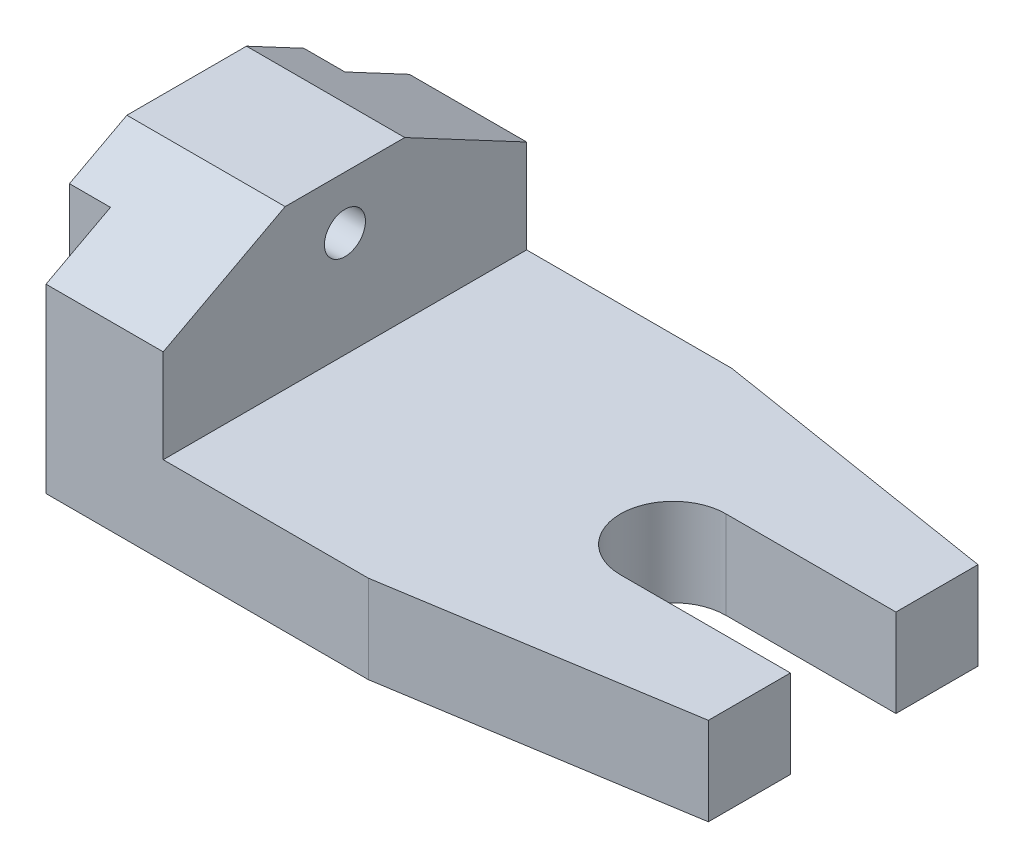
ISO-10303-21;
HEADER;
FILE_DESCRIPTION(('STEP AP214'),'2;1');
FILE_NAME('part.step','',(''),(''),'','','');
FILE_SCHEMA(('AUTOMOTIVE_DESIGN { 1 0 10303 214 1 1 1 1 }'));
ENDSEC;
DATA;
#1=APPLICATION_CONTEXT('core data for automotive mechanical design processes');
#2=APPLICATION_PROTOCOL_DEFINITION('international standard','automotive_design',2000,#1);
#3=PRODUCT_CONTEXT('',#1,'mechanical');
#4=PRODUCT('Part','Part','',(#3));
#5=PRODUCT_RELATED_PRODUCT_CATEGORY('part','',(#4));
#6=PRODUCT_DEFINITION_FORMATION('','',#4);
#7=PRODUCT_DEFINITION_CONTEXT('part definition',#1,'design');
#8=PRODUCT_DEFINITION('design','',#6,#7);
#9=PRODUCT_DEFINITION_SHAPE('','',#8);
#10=(LENGTH_UNIT() NAMED_UNIT(*) SI_UNIT(.MILLI.,.METRE.));
#11=(NAMED_UNIT(*) PLANE_ANGLE_UNIT() SI_UNIT($,.RADIAN.));
#12=(NAMED_UNIT(*) SI_UNIT($,.STERADIAN.) SOLID_ANGLE_UNIT());
#13=UNCERTAINTY_MEASURE_WITH_UNIT(LENGTH_MEASURE(1.E-05),#10,'distance_accuracy_value','');
#14=(GEOMETRIC_REPRESENTATION_CONTEXT(3) GLOBAL_UNCERTAINTY_ASSIGNED_CONTEXT((#13)) GLOBAL_UNIT_ASSIGNED_CONTEXT((#10,
#11,#12)) REPRESENTATION_CONTEXT('',''));
#15=CARTESIAN_POINT('',(0.,0.,0.));
#16=DIRECTION('',(0.,0.,1.));
#17=DIRECTION('',(1.,0.,0.));
#18=AXIS2_PLACEMENT_3D('',#15,#16,#17);
#19=CARTESIAN_POINT('',(112.,0.,31.));
#20=DIRECTION('',(-1.,0.,0.));
#21=DIRECTION('',(0.,0.,1.));
#22=AXIS2_PLACEMENT_3D('',#19,#20,#21);
#23=PLANE('',#22);
#24=DIRECTION('',(0.,0.,-1.));
#25=VECTOR('',#24,1.);
#26=CARTESIAN_POINT('',(112.,15.,31.));
#27=LINE('',#26,#25);
#28=CARTESIAN_POINT('',(112.,15.,23.));
#29=VERTEX_POINT('',#28);
#30=CARTESIAN_POINT('',(112.,15.,9.));
#31=VERTEX_POINT('',#30);
#32=EDGE_CURVE('E177',#29,#31,#27,.T.);
#33=ORIENTED_EDGE('',*,*,#32,.F.);
#34=DIRECTION('',(0.,1.,0.));
#35=VECTOR('',#34,1.);
#36=CARTESIAN_POINT('',(112.,-87.,23.));
#37=LINE('',#36,#35);
#38=CARTESIAN_POINT('',(112.,0.,23.));
#39=VERTEX_POINT('',#38);
#40=EDGE_CURVE('E165',#39,#29,#37,.T.);
#41=ORIENTED_EDGE('',*,*,#40,.F.);
#42=DIRECTION('',(0.,0.,-1.));
#43=VECTOR('',#42,1.);
#44=CARTESIAN_POINT('',(112.,0.,31.));
#45=LINE('',#44,#43);
#46=CARTESIAN_POINT('',(112.,0.,9.));
#47=VERTEX_POINT('',#46);
#48=EDGE_CURVE('E188',#39,#47,#45,.T.);
#49=ORIENTED_EDGE('',*,*,#48,.T.);
#50=DIRECTION('',(0.,1.,0.));
#51=VECTOR('',#50,1.);
#52=CARTESIAN_POINT('',(112.,-87.,9.));
#53=LINE('',#52,#51);
#54=EDGE_CURVE('E184',#47,#31,#53,.T.);
#55=ORIENTED_EDGE('',*,*,#54,.T.);
#56=EDGE_LOOP('',(#33,#41,#49,#55));
#57=FACE_BOUND('',#56,.T.);
#58=ADVANCED_FACE('F41',(#57),#23,.F.);
#59=CARTESIAN_POINT('',(0.,0.,31.));
#60=DIRECTION('',(0.,1.,0.));
#61=DIRECTION('',(0.,0.,1.));
#62=AXIS2_PLACEMENT_3D('',#59,#60,#61);
#63=PLANE('',#62);
#64=ORIENTED_EDGE('',*,*,#48,.F.);
#65=DIRECTION('',(-0.987440631916705,0.,0.157990501106673));
#66=VECTOR('',#65,1.);
#67=CARTESIAN_POINT('',(1.54758190327613,0.,40.6723868954758));
#68=LINE('',#67,#66);
#69=CARTESIAN_POINT('',(62.,0.,31.));
#70=VERTEX_POINT('',#69);
#71=EDGE_CURVE('E170',#39,#70,#68,.T.);
#72=ORIENTED_EDGE('',*,*,#71,.T.);
#73=DIRECTION('',(1.,0.,0.));
#74=VECTOR('',#73,1.);
#75=CARTESIAN_POINT('',(0.,0.,31.));
#76=LINE('',#75,#74);
#77=CARTESIAN_POINT('',(7.,0.,31.));
#78=VERTEX_POINT('',#77);
#79=EDGE_CURVE('E250',#78,#70,#76,.T.);
#80=ORIENTED_EDGE('',*,*,#79,.F.);
#81=DIRECTION('',(0.,0.,-1.));
#82=VECTOR('',#81,1.);
#83=CARTESIAN_POINT('',(7.,0.,31.));
#84=LINE('',#83,#82);
#85=CARTESIAN_POINT('',(7.,0.,20.));
#86=VERTEX_POINT('',#85);
#87=EDGE_CURVE('E297',#78,#86,#84,.T.);
#88=ORIENTED_EDGE('',*,*,#87,.T.);
#89=DIRECTION('',(-1.,0.,0.));
#90=VECTOR('',#89,1.);
#91=CARTESIAN_POINT('',(0.,0.,20.));
#92=LINE('',#91,#90);
#93=CARTESIAN_POINT('',(0.,0.,20.));
#94=VERTEX_POINT('',#93);
#95=EDGE_CURVE('E314',#86,#94,#92,.T.);
#96=ORIENTED_EDGE('',*,*,#95,.T.);
#97=DIRECTION('',(0.,0.,-1.));
#98=VECTOR('',#97,1.);
#99=CARTESIAN_POINT('',(0.,0.,31.));
#100=LINE('',#99,#98);
#101=CARTESIAN_POINT('',(0.,0.,-20.));
#102=VERTEX_POINT('',#101);
#103=EDGE_CURVE('E247',#94,#102,#100,.T.);
#104=ORIENTED_EDGE('',*,*,#103,.T.);
#105=DIRECTION('',(1.,0.,0.));
#106=VECTOR('',#105,1.);
#107=CARTESIAN_POINT('',(0.,0.,-20.));
#108=LINE('',#107,#106);
#109=CARTESIAN_POINT('',(7.,0.,-20.));
#110=VERTEX_POINT('',#109);
#111=EDGE_CURVE('E319',#102,#110,#108,.T.);
#112=ORIENTED_EDGE('',*,*,#111,.T.);
#113=DIRECTION('',(0.,0.,-1.));
#114=VECTOR('',#113,1.);
#115=CARTESIAN_POINT('',(7.00000000000002,0.,31.));
#116=LINE('',#115,#114);
#117=CARTESIAN_POINT('',(7.,0.,-31.));
#118=VERTEX_POINT('',#117);
#119=EDGE_CURVE('E232',#110,#118,#116,.T.);
#120=ORIENTED_EDGE('',*,*,#119,.T.);
#121=DIRECTION('',(1.,0.,0.));
#122=VECTOR('',#121,1.);
#123=CARTESIAN_POINT('',(0.,0.,-31.));
#124=LINE('',#123,#122);
#125=CARTESIAN_POINT('',(62.,0.,-31.));
#126=VERTEX_POINT('',#125);
#127=EDGE_CURVE('E224',#118,#126,#124,.T.);
#128=ORIENTED_EDGE('',*,*,#127,.T.);
#129=DIRECTION('',(0.987440631916706,0.,0.157990501106673));
#130=VECTOR('',#129,1.);
#131=CARTESIAN_POINT('',(11.2199687987519,0.,-39.1248049921997));
#132=LINE('',#131,#130);
#133=CARTESIAN_POINT('',(112.,0.,-23.));
#134=VERTEX_POINT('',#133);
#135=EDGE_CURVE('E175',#126,#134,#132,.T.);
#136=ORIENTED_EDGE('',*,*,#135,.T.);
#137=CARTESIAN_POINT('',(112.,0.,-9.));
#138=VERTEX_POINT('',#137);
#139=EDGE_CURVE('E187',#138,#134,#45,.T.);
#140=ORIENTED_EDGE('',*,*,#139,.F.);
#141=DIRECTION('',(-1.,0.,0.));
#142=VECTOR('',#141,1.);
#143=CARTESIAN_POINT('',(0.,0.,-8.99999999999999));
#144=LINE('',#143,#142);
#145=CARTESIAN_POINT('',(83.,0.,-9.));
#146=VERTEX_POINT('',#145);
#147=EDGE_CURVE('E288',#138,#146,#144,.T.);
#148=ORIENTED_EDGE('',*,*,#147,.T.);
#149=CARTESIAN_POINT('',(83.,0.,0.));
#150=DIRECTION('',(0.,1.,0.));
#151=DIRECTION('',(0.,0.,1.));
#152=AXIS2_PLACEMENT_3D('',#149,#150,#151);
#153=CIRCLE('',#152,9.);
#154=CARTESIAN_POINT('',(83.,0.,9.));
#155=VERTEX_POINT('',#154);
#156=EDGE_CURVE('E293',#146,#155,#153,.T.);
#157=ORIENTED_EDGE('',*,*,#156,.T.);
#158=DIRECTION('',(1.,0.,0.));
#159=VECTOR('',#158,1.);
#160=CARTESIAN_POINT('',(0.,0.,9.));
#161=LINE('',#160,#159);
#162=EDGE_CURVE('E295',#155,#47,#161,.T.);
#163=ORIENTED_EDGE('',*,*,#162,.T.);
#164=EDGE_LOOP('',(#64,#72,#80,#88,#96,#104,#112,#120,#128,#136,#140,#148,#157,#163));
#165=FACE_BOUND('',#164,.T.);
#166=ADVANCED_FACE('F43',(#165),#63,.F.);
#167=ORIENTED_EDGE('',*,*,#139,.T.);
#168=DIRECTION('',(0.,1.,0.));
#169=VECTOR('',#168,1.);
#170=CARTESIAN_POINT('',(112.,-87.,-23.));
#171=LINE('',#170,#169);
#172=CARTESIAN_POINT('',(112.,15.,-23.));
#173=VERTEX_POINT('',#172);
#174=EDGE_CURVE('E269',#134,#173,#171,.T.);
#175=ORIENTED_EDGE('',*,*,#174,.T.);
#176=CARTESIAN_POINT('',(112.,15.,-9.));
#177=VERTEX_POINT('',#176);
#178=EDGE_CURVE('E190',#177,#173,#27,.T.);
#179=ORIENTED_EDGE('',*,*,#178,.F.);
#180=DIRECTION('',(0.,1.,0.));
#181=VECTOR('',#180,1.);
#182=CARTESIAN_POINT('',(112.,-87.,-9.));
#183=LINE('',#182,#181);
#184=EDGE_CURVE('E57',#138,#177,#183,.T.);
#185=ORIENTED_EDGE('',*,*,#184,.F.);
#186=EDGE_LOOP('',(#167,#175,#179,#185));
#187=FACE_BOUND('',#186,.T.);
#188=ADVANCED_FACE('F350',(#187),#23,.F.);
#189=CARTESIAN_POINT('',(0.,15.,31.));
#190=DIRECTION('',(0.,1.,0.));
#191=DIRECTION('',(0.,0.,1.));
#192=AXIS2_PLACEMENT_3D('',#189,#190,#191);
#193=PLANE('',#192);
#194=DIRECTION('',(-0.987440631916705,0.,0.157990501106673));
#195=VECTOR('',#194,1.);
#196=CARTESIAN_POINT('',(62.,15.,31.));
#197=LINE('',#196,#195);
#198=CARTESIAN_POINT('',(62.,15.,31.));
#199=VERTEX_POINT('',#198);
#200=EDGE_CURVE('E64',#29,#199,#197,.T.);
#201=ORIENTED_EDGE('',*,*,#200,.F.);
#202=ORIENTED_EDGE('',*,*,#32,.T.);
#203=DIRECTION('',(1.,0.,0.));
#204=VECTOR('',#203,1.);
#205=CARTESIAN_POINT('',(83.,15.,9.));
#206=LINE('',#205,#204);
#207=CARTESIAN_POINT('',(83.,15.,9.));
#208=VERTEX_POINT('',#207);
#209=EDGE_CURVE('E273',#208,#31,#206,.T.);
#210=ORIENTED_EDGE('',*,*,#209,.F.);
#211=CARTESIAN_POINT('',(83.,15.,0.));
#212=DIRECTION('',(0.,1.,0.));
#213=DIRECTION('',(0.,0.,1.));
#214=AXIS2_PLACEMENT_3D('',#211,#212,#213);
#215=CIRCLE('',#214,9.);
#216=CARTESIAN_POINT('',(83.,15.,-9.));
#217=VERTEX_POINT('',#216);
#218=EDGE_CURVE('E285',#217,#208,#215,.T.);
#219=ORIENTED_EDGE('',*,*,#218,.F.);
#220=DIRECTION('',(-1.,0.,0.));
#221=VECTOR('',#220,1.);
#222=CARTESIAN_POINT('',(83.,15.,-9.));
#223=LINE('',#222,#221);
#224=EDGE_CURVE('E272',#177,#217,#223,.T.);
#225=ORIENTED_EDGE('',*,*,#224,.F.);
#226=ORIENTED_EDGE('',*,*,#178,.T.);
#227=DIRECTION('',(0.987440631916705,0.,0.157990501106673));
#228=VECTOR('',#227,1.);
#229=CARTESIAN_POINT('',(62.,15.,-31.));
#230=LINE('',#229,#228);
#231=CARTESIAN_POINT('',(62.,15.,-31.));
#232=VERTEX_POINT('',#231);
#233=EDGE_CURVE('E185',#232,#173,#230,.T.);
#234=ORIENTED_EDGE('',*,*,#233,.F.);
#235=DIRECTION('',(1.,0.,0.));
#236=VECTOR('',#235,1.);
#237=CARTESIAN_POINT('',(0.,15.,-31.));
#238=LINE('',#237,#236);
#239=CARTESIAN_POINT('',(27.,15.,-31.));
#240=VERTEX_POINT('',#239);
#241=EDGE_CURVE('E227',#240,#232,#238,.T.);
#242=ORIENTED_EDGE('',*,*,#241,.F.);
#243=DIRECTION('',(0.,0.,-1.));
#244=VECTOR('',#243,1.);
#245=CARTESIAN_POINT('',(27.,15.,31.));
#246=LINE('',#245,#244);
#247=CARTESIAN_POINT('',(27.,15.,31.));
#248=VERTEX_POINT('',#247);
#249=EDGE_CURVE('E194',#248,#240,#246,.T.);
#250=ORIENTED_EDGE('',*,*,#249,.F.);
#251=DIRECTION('',(1.,0.,0.));
#252=VECTOR('',#251,1.);
#253=CARTESIAN_POINT('',(0.,15.,31.));
#254=LINE('',#253,#252);
#255=EDGE_CURVE('E181',#248,#199,#254,.T.);
#256=ORIENTED_EDGE('',*,*,#255,.T.);
#257=EDGE_LOOP('',(#201,#202,#210,#219,#225,#226,#234,#242,#250,#256));
#258=FACE_BOUND('',#257,.T.);
#259=ADVANCED_FACE('F180',(#258),#193,.T.);
#260=CARTESIAN_POINT('',(27.,0.,31.));
#261=DIRECTION('',(-1.,0.,0.));
#262=DIRECTION('',(0.,0.,1.));
#263=AXIS2_PLACEMENT_3D('',#260,#261,#262);
#264=PLANE('',#263);
#265=CARTESIAN_POINT('',(27.,33.,0.));
#266=DIRECTION('',(-1.,0.,0.));
#267=DIRECTION('',(0.,0.,1.));
#268=AXIS2_PLACEMENT_3D('',#265,#266,#267);
#269=CIRCLE('',#268,3.5);
#270=CARTESIAN_POINT('',(27.,33.,3.5));
#271=VERTEX_POINT('',#270);
#272=EDGE_CURVE('E201',#271,#271,#269,.T.);
#273=ORIENTED_EDGE('',*,*,#272,.T.);
#274=EDGE_LOOP('',(#273));
#275=FACE_BOUND('',#274,.T.);
#276=DIRECTION('',(0.,0.,-1.));
#277=VECTOR('',#276,1.);
#278=CARTESIAN_POINT('',(27.,42.,31.));
#279=LINE('',#278,#277);
#280=CARTESIAN_POINT('',(27.,42.,10.2));
#281=VERTEX_POINT('',#280);
#282=CARTESIAN_POINT('',(27.,42.,-10.2029798390233));
#283=VERTEX_POINT('',#282);
#284=EDGE_CURVE('E254',#281,#283,#279,.T.);
#285=ORIENTED_EDGE('',*,*,#284,.F.);
#286=DIRECTION('',(0.,-0.469471562785885,0.88294759285893));
#287=VECTOR('',#286,1.);
#288=CARTESIAN_POINT('',(27.,24.1210602183135,43.8253952197516));
#289=LINE('',#288,#287);
#290=CARTESIAN_POINT('',(27.,30.9404438214414,31.));
#291=VERTEX_POINT('',#290);
#292=EDGE_CURVE('E207',#281,#291,#289,.T.);
#293=ORIENTED_EDGE('',*,*,#292,.T.);
#294=DIRECTION('',(0.,1.,0.));
#295=VECTOR('',#294,1.);
#296=CARTESIAN_POINT('',(27.,0.,31.));
#297=LINE('',#296,#295);
#298=EDGE_CURVE('E245',#248,#291,#297,.T.);
#299=ORIENTED_EDGE('',*,*,#298,.F.);
#300=ORIENTED_EDGE('',*,*,#249,.T.);
#301=DIRECTION('',(0.,1.,0.));
#302=VECTOR('',#301,1.);
#303=CARTESIAN_POINT('',(27.,0.,-31.));
#304=LINE('',#303,#302);
#305=CARTESIAN_POINT('',(27.,30.9420282299548,-31.));
#306=VERTEX_POINT('',#305);
#307=EDGE_CURVE('E240',#240,#306,#304,.T.);
#308=ORIENTED_EDGE('',*,*,#307,.T.);
#309=DIRECTION('',(0.,0.469471562785892,0.882947592858926));
#310=VECTOR('',#309,1.);
#311=CARTESIAN_POINT('',(27.,49.8224601667748,4.50892802074745));
#312=LINE('',#311,#310);
#313=EDGE_CURVE('E330',#306,#283,#312,.T.);
#314=ORIENTED_EDGE('',*,*,#313,.T.);
#315=EDGE_LOOP('',(#285,#293,#299,#300,#308,#314));
#316=FACE_BOUND('',#315,.T.);
#317=ADVANCED_FACE('F262',(#275,#316),#264,.F.);
#318=CARTESIAN_POINT('',(0.,42.,31.));
#319=DIRECTION('',(0.,1.,0.));
#320=DIRECTION('',(0.,0.,1.));
#321=AXIS2_PLACEMENT_3D('',#318,#319,#320);
#322=PLANE('',#321);
#323=DIRECTION('',(1.,0.,0.));
#324=VECTOR('',#323,1.);
#325=CARTESIAN_POINT('',(-4.,42.,10.2));
#326=LINE('',#325,#324);
#327=CARTESIAN_POINT('',(0.,42.,10.2));
#328=VERTEX_POINT('',#327);
#329=EDGE_CURVE('E322',#328,#281,#326,.T.);
#330=ORIENTED_EDGE('',*,*,#329,.T.);
#331=ORIENTED_EDGE('',*,*,#284,.T.);
#332=DIRECTION('',(1.,0.,0.));
#333=VECTOR('',#332,1.);
#334=CARTESIAN_POINT('',(-4.,42.,-10.2029798390233));
#335=LINE('',#334,#333);
#336=CARTESIAN_POINT('',(0.,42.,-10.2029798390233));
#337=VERTEX_POINT('',#336);
#338=EDGE_CURVE('E325',#337,#283,#335,.T.);
#339=ORIENTED_EDGE('',*,*,#338,.F.);
#340=DIRECTION('',(0.,0.,-1.));
#341=VECTOR('',#340,1.);
#342=CARTESIAN_POINT('',(0.,42.,31.));
#343=LINE('',#342,#341);
#344=EDGE_CURVE('E252',#328,#337,#343,.T.);
#345=ORIENTED_EDGE('',*,*,#344,.F.);
#346=EDGE_LOOP('',(#330,#331,#339,#345));
#347=FACE_BOUND('',#346,.T.);
#348=ADVANCED_FACE('F374',(#347),#322,.T.);
#349=CARTESIAN_POINT('',(0.,0.,31.));
#350=DIRECTION('',(-1.,0.,0.));
#351=DIRECTION('',(0.,0.,1.));
#352=AXIS2_PLACEMENT_3D('',#349,#350,#351);
#353=PLANE('',#352);
#354=DIRECTION('',(0.,1.,0.));
#355=VECTOR('',#354,1.);
#356=CARTESIAN_POINT('',(0.,-8.99999999999998,-20.));
#357=LINE('',#356,#355);
#358=CARTESIAN_POINT('',(0.,36.790831978231,-20.));
#359=VERTEX_POINT('',#358);
#360=EDGE_CURVE('E302',#102,#359,#357,.T.);
#361=ORIENTED_EDGE('',*,*,#360,.F.);
#362=ORIENTED_EDGE('',*,*,#103,.F.);
#363=DIRECTION('',(0.,1.,0.));
#364=VECTOR('',#363,1.);
#365=CARTESIAN_POINT('',(0.,-8.99999999999998,20.));
#366=LINE('',#365,#364);
#367=CARTESIAN_POINT('',(0.,36.7892475697176,20.));
#368=VERTEX_POINT('',#367);
#369=EDGE_CURVE('E300',#94,#368,#366,.T.);
#370=ORIENTED_EDGE('',*,*,#369,.T.);
#371=DIRECTION('',(0.,-0.469471562785885,0.88294759285893));
#372=VECTOR('',#371,1.);
#373=CARTESIAN_POINT('',(0.,24.1210602183135,43.8253952197516));
#374=LINE('',#373,#372);
#375=EDGE_CURVE('E326',#328,#368,#374,.T.);
#376=ORIENTED_EDGE('',*,*,#375,.F.);
#377=ORIENTED_EDGE('',*,*,#344,.T.);
#378=DIRECTION('',(0.,0.469471562785892,0.882947592858926));
#379=VECTOR('',#378,1.);
#380=CARTESIAN_POINT('',(0.,49.8224601667748,4.50892802074745));
#381=LINE('',#380,#379);
#382=EDGE_CURVE('E321',#359,#337,#381,.T.);
#383=ORIENTED_EDGE('',*,*,#382,.F.);
#384=EDGE_LOOP('',(#361,#362,#370,#376,#377,#383));
#385=FACE_BOUND('',#384,.T.);
#386=CARTESIAN_POINT('',(0.,33.,0.));
#387=DIRECTION('',(-1.,0.,0.));
#388=DIRECTION('',(0.,0.,1.));
#389=AXIS2_PLACEMENT_3D('',#386,#387,#388);
#390=CIRCLE('',#389,3.5);
#391=CARTESIAN_POINT('',(0.,33.,3.5));
#392=VERTEX_POINT('',#391);
#393=EDGE_CURVE('E205',#392,#392,#390,.T.);
#394=ORIENTED_EDGE('',*,*,#393,.F.);
#395=EDGE_LOOP('',(#394));
#396=FACE_BOUND('',#395,.T.);
#397=ADVANCED_FACE('F382',(#385,#396),#353,.T.);
#398=CARTESIAN_POINT('',(0.,0.,31.));
#399=DIRECTION('',(0.,0.,1.));
#400=DIRECTION('',(1.,0.,0.));
#401=AXIS2_PLACEMENT_3D('',#398,#399,#400);
#402=PLANE('',#401);
#403=DIRECTION('',(0.,-1.,0.));
#404=VECTOR('',#403,1.);
#405=CARTESIAN_POINT('',(62.,0.,31.));
#406=LINE('',#405,#404);
#407=EDGE_CURVE('E11',#199,#70,#406,.T.);
#408=ORIENTED_EDGE('',*,*,#407,.F.);
#409=ORIENTED_EDGE('',*,*,#255,.F.);
#410=ORIENTED_EDGE('',*,*,#298,.T.);
#411=DIRECTION('',(1.,0.,0.));
#412=VECTOR('',#411,1.);
#413=CARTESIAN_POINT('',(0.,30.9404438214414,31.));
#414=LINE('',#413,#412);
#415=CARTESIAN_POINT('',(7.,30.9404438214414,31.));
#416=VERTEX_POINT('',#415);
#417=EDGE_CURVE('E196',#416,#291,#414,.T.);
#418=ORIENTED_EDGE('',*,*,#417,.F.);
#419=DIRECTION('',(0.,1.,0.));
#420=VECTOR('',#419,1.);
#421=CARTESIAN_POINT('',(7.,-8.99999999999998,31.));
#422=LINE('',#421,#420);
#423=EDGE_CURVE('E306',#78,#416,#422,.T.);
#424=ORIENTED_EDGE('',*,*,#423,.F.);
#425=ORIENTED_EDGE('',*,*,#79,.T.);
#426=EDGE_LOOP('',(#408,#409,#410,#418,#424,#425));
#427=FACE_BOUND('',#426,.T.);
#428=ADVANCED_FACE('F337',(#427),#402,.T.);
#429=CARTESIAN_POINT('',(0.,0.,-31.));
#430=DIRECTION('',(0.,0.,1.));
#431=DIRECTION('',(1.,0.,0.));
#432=AXIS2_PLACEMENT_3D('',#429,#430,#431);
#433=PLANE('',#432);
#434=ORIENTED_EDGE('',*,*,#241,.T.);
#435=DIRECTION('',(0.,-1.,0.));
#436=VECTOR('',#435,1.);
#437=CARTESIAN_POINT('',(62.,0.,-31.));
#438=LINE('',#437,#436);
#439=EDGE_CURVE('E47',#232,#126,#438,.T.);
#440=ORIENTED_EDGE('',*,*,#439,.T.);
#441=ORIENTED_EDGE('',*,*,#127,.F.);
#442=DIRECTION('',(0.,1.,0.));
#443=VECTOR('',#442,1.);
#444=CARTESIAN_POINT('',(7.,-8.99999999999998,-31.));
#445=LINE('',#444,#443);
#446=CARTESIAN_POINT('',(7.,30.9420282299548,-31.));
#447=VERTEX_POINT('',#446);
#448=EDGE_CURVE('E296',#118,#447,#445,.T.);
#449=ORIENTED_EDGE('',*,*,#448,.T.);
#450=DIRECTION('',(1.,0.,0.));
#451=VECTOR('',#450,1.);
#452=CARTESIAN_POINT('',(0.,30.9420282299548,-31.));
#453=LINE('',#452,#451);
#454=EDGE_CURVE('E200',#447,#306,#453,.T.);
#455=ORIENTED_EDGE('',*,*,#454,.T.);
#456=ORIENTED_EDGE('',*,*,#307,.F.);
#457=EDGE_LOOP('',(#434,#440,#441,#449,#455,#456));
#458=FACE_BOUND('',#457,.T.);
#459=ADVANCED_FACE('F225',(#458),#433,.F.);
#460=CARTESIAN_POINT('',(-4.,42.,-10.2029798390233));
#461=DIRECTION('',(0.,-0.882947592858926,0.469471562785892));
#462=DIRECTION('',(0.,-0.469471562785892,-0.882947592858926));
#463=AXIS2_PLACEMENT_3D('',#460,#461,#462);
#464=PLANE('',#463);
#465=ORIENTED_EDGE('',*,*,#454,.F.);
#466=DIRECTION('',(0.,0.469471562785892,0.882947592858926));
#467=VECTOR('',#466,1.);
#468=CARTESIAN_POINT('',(7.,42.,-10.2029798390233));
#469=LINE('',#468,#467);
#470=CARTESIAN_POINT('',(7.,36.790831978231,-20.));
#471=VERTEX_POINT('',#470);
#472=EDGE_CURVE('E213',#447,#471,#469,.T.);
#473=ORIENTED_EDGE('',*,*,#472,.T.);
#474=DIRECTION('',(-1.,0.,0.));
#475=VECTOR('',#474,1.);
#476=CARTESIAN_POINT('',(-4.,36.790831978231,-20.));
#477=LINE('',#476,#475);
#478=EDGE_CURVE('E215',#471,#359,#477,.T.);
#479=ORIENTED_EDGE('',*,*,#478,.T.);
#480=ORIENTED_EDGE('',*,*,#382,.T.);
#481=ORIENTED_EDGE('',*,*,#338,.T.);
#482=ORIENTED_EDGE('',*,*,#313,.F.);
#483=EDGE_LOOP('',(#465,#473,#479,#480,#481,#482));
#484=FACE_BOUND('',#483,.T.);
#485=ADVANCED_FACE('F387',(#484),#464,.F.);
#486=CARTESIAN_POINT('',(-4.,42.,10.2));
#487=DIRECTION('',(0.,-0.88294759285893,-0.469471562785885));
#488=DIRECTION('',(0.,0.469471562785885,-0.88294759285893));
#489=AXIS2_PLACEMENT_3D('',#486,#487,#488);
#490=PLANE('',#489);
#491=ORIENTED_EDGE('',*,*,#375,.T.);
#492=DIRECTION('',(1.,0.,0.));
#493=VECTOR('',#492,1.);
#494=CARTESIAN_POINT('',(-4.,36.7892475697176,20.));
#495=LINE('',#494,#493);
#496=CARTESIAN_POINT('',(7.,36.7892475697176,20.));
#497=VERTEX_POINT('',#496);
#498=EDGE_CURVE('E209',#368,#497,#495,.T.);
#499=ORIENTED_EDGE('',*,*,#498,.T.);
#500=DIRECTION('',(0.,-0.469471562785885,0.88294759285893));
#501=VECTOR('',#500,1.);
#502=CARTESIAN_POINT('',(7.,42.,10.2));
#503=LINE('',#502,#501);
#504=EDGE_CURVE('E202',#497,#416,#503,.T.);
#505=ORIENTED_EDGE('',*,*,#504,.T.);
#506=ORIENTED_EDGE('',*,*,#417,.T.);
#507=ORIENTED_EDGE('',*,*,#292,.F.);
#508=ORIENTED_EDGE('',*,*,#329,.F.);
#509=EDGE_LOOP('',(#491,#499,#505,#506,#507,#508));
#510=FACE_BOUND('',#509,.T.);
#511=ADVANCED_FACE('F395',(#510),#490,.F.);
#512=CARTESIAN_POINT('',(-4.,33.,0.));
#513=DIRECTION('',(1.,0.,0.));
#514=DIRECTION('',(0.,0.,-1.));
#515=AXIS2_PLACEMENT_3D('',#512,#513,#514);
#516=CYLINDRICAL_SURFACE('',#515,3.5);
#517=ORIENTED_EDGE('',*,*,#393,.T.);
#518=EDGE_LOOP('',(#517));
#519=FACE_BOUND('',#518,.T.);
#520=ORIENTED_EDGE('',*,*,#272,.F.);
#521=EDGE_LOOP('',(#520));
#522=FACE_BOUND('',#521,.T.);
#523=ADVANCED_FACE('F389',(#519,#522),#516,.F.);
#524=CARTESIAN_POINT('',(0.,-8.99999999999998,20.));
#525=DIRECTION('',(0.,0.,-1.));
#526=DIRECTION('',(-1.,0.,0.));
#527=AXIS2_PLACEMENT_3D('',#524,#525,#526);
#528=PLANE('',#527);
#529=DIRECTION('',(0.,1.,0.));
#530=VECTOR('',#529,1.);
#531=CARTESIAN_POINT('',(7.,-8.99999999999998,20.));
#532=LINE('',#531,#530);
#533=EDGE_CURVE('E308',#86,#497,#532,.T.);
#534=ORIENTED_EDGE('',*,*,#533,.T.);
#535=ORIENTED_EDGE('',*,*,#498,.F.);
#536=ORIENTED_EDGE('',*,*,#369,.F.);
#537=ORIENTED_EDGE('',*,*,#95,.F.);
#538=EDGE_LOOP('',(#534,#535,#536,#537));
#539=FACE_BOUND('',#538,.T.);
#540=ADVANCED_FACE('F392',(#539),#528,.F.);
#541=CARTESIAN_POINT('',(7.,-8.99999999999998,31.));
#542=DIRECTION('',(1.,0.,0.));
#543=DIRECTION('',(0.,0.,-1.));
#544=AXIS2_PLACEMENT_3D('',#541,#542,#543);
#545=PLANE('',#544);
#546=ORIENTED_EDGE('',*,*,#423,.T.);
#547=ORIENTED_EDGE('',*,*,#504,.F.);
#548=ORIENTED_EDGE('',*,*,#533,.F.);
#549=ORIENTED_EDGE('',*,*,#87,.F.);
#550=EDGE_LOOP('',(#546,#547,#548,#549));
#551=FACE_BOUND('',#550,.T.);
#552=ADVANCED_FACE('F405',(#551),#545,.F.);
#553=CARTESIAN_POINT('',(7.,-8.99999999999998,-31.));
#554=DIRECTION('',(1.,0.,0.));
#555=DIRECTION('',(0.,0.,-1.));
#556=AXIS2_PLACEMENT_3D('',#553,#554,#555);
#557=PLANE('',#556);
#558=DIRECTION('',(0.,1.,0.));
#559=VECTOR('',#558,1.);
#560=CARTESIAN_POINT('',(7.,-8.99999999999998,-20.));
#561=LINE('',#560,#559);
#562=EDGE_CURVE('E301',#110,#471,#561,.T.);
#563=ORIENTED_EDGE('',*,*,#562,.T.);
#564=ORIENTED_EDGE('',*,*,#472,.F.);
#565=ORIENTED_EDGE('',*,*,#448,.F.);
#566=ORIENTED_EDGE('',*,*,#119,.F.);
#567=EDGE_LOOP('',(#563,#564,#565,#566));
#568=FACE_BOUND('',#567,.T.);
#569=ADVANCED_FACE('F356',(#568),#557,.F.);
#570=CARTESIAN_POINT('',(0.,-8.99999999999998,-20.));
#571=DIRECTION('',(0.,0.,1.));
#572=DIRECTION('',(1.,0.,0.));
#573=AXIS2_PLACEMENT_3D('',#570,#571,#572);
#574=PLANE('',#573);
#575=ORIENTED_EDGE('',*,*,#360,.T.);
#576=ORIENTED_EDGE('',*,*,#478,.F.);
#577=ORIENTED_EDGE('',*,*,#562,.F.);
#578=ORIENTED_EDGE('',*,*,#111,.F.);
#579=EDGE_LOOP('',(#575,#576,#577,#578));
#580=FACE_BOUND('',#579,.T.);
#581=ADVANCED_FACE('F348',(#580),#574,.F.);
#582=CARTESIAN_POINT('',(62.,-87.,-31.));
#583=DIRECTION('',(-0.157990501106673,0.,0.987440631916705));
#584=DIRECTION('',(0.987440631916706,0.,0.157990501106673));
#585=AXIS2_PLACEMENT_3D('',#582,#583,#584);
#586=PLANE('',#585);
#587=ORIENTED_EDGE('',*,*,#439,.F.);
#588=ORIENTED_EDGE('',*,*,#233,.T.);
#589=ORIENTED_EDGE('',*,*,#174,.F.);
#590=ORIENTED_EDGE('',*,*,#135,.F.);
#591=EDGE_LOOP('',(#587,#588,#589,#590));
#592=FACE_BOUND('',#591,.T.);
#593=ADVANCED_FACE('F349',(#592),#586,.F.);
#594=CARTESIAN_POINT('',(62.,-87.,31.));
#595=DIRECTION('',(-0.157990501106673,0.,-0.987440631916706));
#596=DIRECTION('',(-0.987440631916705,0.,0.157990501106673));
#597=AXIS2_PLACEMENT_3D('',#594,#595,#596);
#598=PLANE('',#597);
#599=ORIENTED_EDGE('',*,*,#40,.T.);
#600=ORIENTED_EDGE('',*,*,#200,.T.);
#601=ORIENTED_EDGE('',*,*,#407,.T.);
#602=ORIENTED_EDGE('',*,*,#71,.F.);
#603=EDGE_LOOP('',(#599,#600,#601,#602));
#604=FACE_BOUND('',#603,.T.);
#605=ADVANCED_FACE('F164',(#604),#598,.F.);
#606=CARTESIAN_POINT('',(83.,-87.,9.));
#607=DIRECTION('',(0.,0.,1.));
#608=DIRECTION('',(1.,0.,0.));
#609=AXIS2_PLACEMENT_3D('',#606,#607,#608);
#610=PLANE('',#609);
#611=DIRECTION('',(0.,1.,0.));
#612=VECTOR('',#611,1.);
#613=CARTESIAN_POINT('',(83.,-87.,9.));
#614=LINE('',#613,#612);
#615=EDGE_CURVE('E279',#155,#208,#614,.T.);
#616=ORIENTED_EDGE('',*,*,#615,.T.);
#617=ORIENTED_EDGE('',*,*,#209,.T.);
#618=ORIENTED_EDGE('',*,*,#54,.F.);
#619=ORIENTED_EDGE('',*,*,#162,.F.);
#620=EDGE_LOOP('',(#616,#617,#618,#619));
#621=FACE_BOUND('',#620,.T.);
#622=ADVANCED_FACE('F342',(#621),#610,.F.);
#623=CARTESIAN_POINT('',(83.,-87.,0.));
#624=DIRECTION('',(0.,1.,0.));
#625=DIRECTION('',(0.,0.,1.));
#626=AXIS2_PLACEMENT_3D('',#623,#624,#625);
#627=CYLINDRICAL_SURFACE('',#626,9.);
#628=DIRECTION('',(0.,1.,0.));
#629=VECTOR('',#628,1.);
#630=CARTESIAN_POINT('',(83.,-87.,-9.));
#631=LINE('',#630,#629);
#632=EDGE_CURVE('E277',#146,#217,#631,.T.);
#633=ORIENTED_EDGE('',*,*,#632,.T.);
#634=ORIENTED_EDGE('',*,*,#218,.T.);
#635=ORIENTED_EDGE('',*,*,#615,.F.);
#636=ORIENTED_EDGE('',*,*,#156,.F.);
#637=EDGE_LOOP('',(#633,#634,#635,#636));
#638=FACE_BOUND('',#637,.T.);
#639=ADVANCED_FACE('F344',(#638),#627,.F.);
#640=CARTESIAN_POINT('',(83.,-87.,-9.));
#641=DIRECTION('',(0.,0.,-1.));
#642=DIRECTION('',(-1.,0.,0.));
#643=AXIS2_PLACEMENT_3D('',#640,#641,#642);
#644=PLANE('',#643);
#645=ORIENTED_EDGE('',*,*,#184,.T.);
#646=ORIENTED_EDGE('',*,*,#224,.T.);
#647=ORIENTED_EDGE('',*,*,#632,.F.);
#648=ORIENTED_EDGE('',*,*,#147,.F.);
#649=EDGE_LOOP('',(#645,#646,#647,#648));
#650=FACE_BOUND('',#649,.T.);
#651=ADVANCED_FACE('F414',(#650),#644,.F.);
#652=CLOSED_SHELL('',(#58,#166,#188,#259,#317,#348,#397,#428,#459,#485,#511,#523,#540,#552,#569,
#581,#593,#605,#622,#639,#651));
#653=MANIFOLD_SOLID_BREP('B2',#652);
#654=ADVANCED_BREP_SHAPE_REPRESENTATION('',(#18,#653),#14);
#655=SHAPE_DEFINITION_REPRESENTATION(#9,#654);
ENDSEC;
END-ISO-10303-21;
